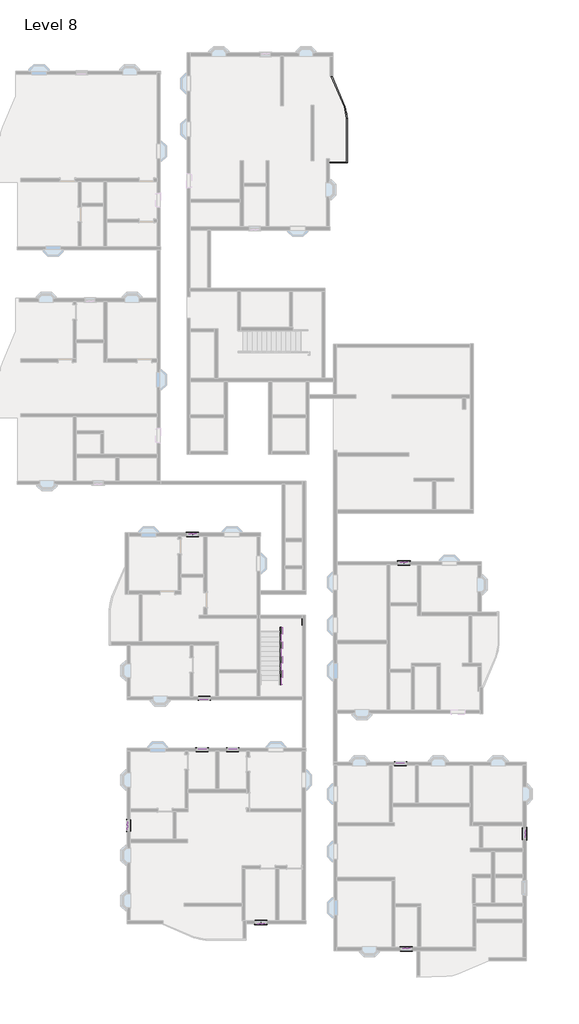
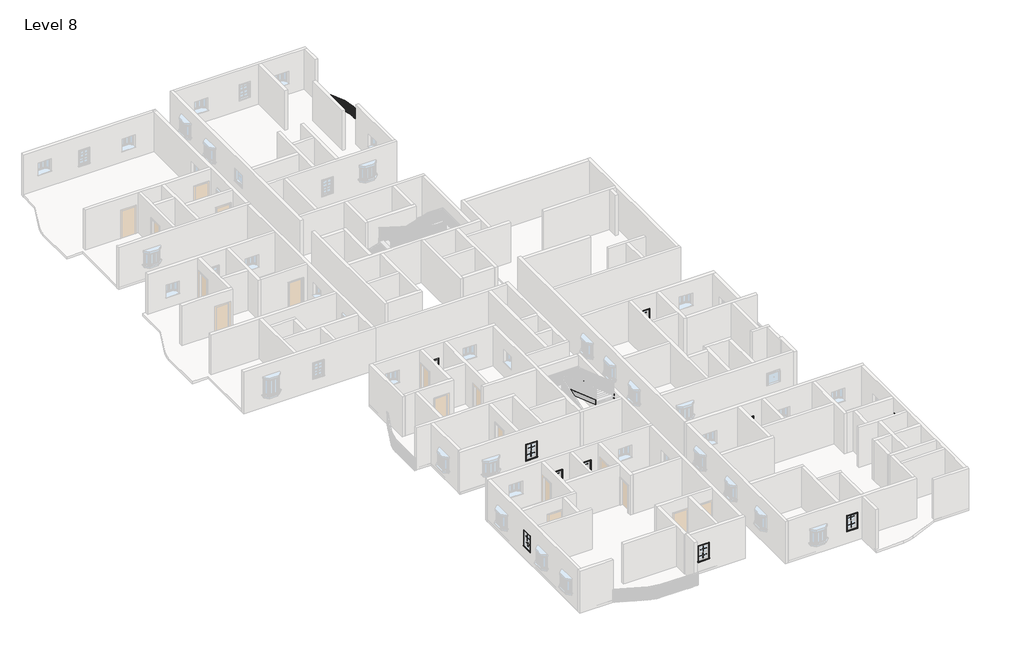
# One storey, part 13 of 14: 40 proxies, 6 members, 1 railing.
"""IFC4 building model written with IfcOpenShell, lengths in millimetres."""

from ifc_helpers import new_model, si_unit, frame, origin, place, context, project, spatial, polyline, circle_curve, outline, extrude, transform, mapped, element, save
from ifc_brep_helpers import plane_surface, cylinder_surface, revolved_surface, advanced_brep
from components import muntin_pattern_2x2_muntin_pattern_2x2_c35c595f, trim_window_exterior_flat_with_sill_e38017c9, trim_window_interior_flat_picture_frame_d728ed12

model = new_model("IFC4")

# Units and contexts
model_context = context("Model", 3, world=origin())
ifc_project = project(units=[si_unit("LENGTHUNIT", "METRE", prefix="MILLI")], contexts=[model_context])

# Site, building, storey
site = spatial("IfcSite", under=ifc_project)
building = spatial("IfcBuilding", under=site)
storey = spatial("IfcBuildingStorey", under=building, Name="Level 8", Elevation=21336.0)

# Proxies
placement = place(None, origin())
muntin_pattern_2x2_muntin_pattern_2x2_shape = muntin_pattern_2x2_muntin_pattern_2x2_c35c595f(model_context)
element("IfcBuildingElementProxy", 1, Name="Muntin Pattern_2x2 : Muntin Pattern_2x2", ObjectType="Muntin Pattern_2x2 : Muntin Pattern_2x2", at=placement, inside=storey, context=model_context, shape_type="MappedRepresentation", body=[
    mapped(muntin_pattern_2x2_muntin_pattern_2x2_shape, transform((-8150.287215, -357.5666506, 22806.025), x_axis=(1.0, 0.0, 0.0), y_axis=(0.0, 1.0, 0.0), z_axis=(0.0, 0.0, 1.0))),
])
element("IfcBuildingElementProxy", 2, Name="Muntin Pattern_2x2 : Muntin Pattern_2x2", ObjectType="Muntin Pattern_2x2 : Muntin Pattern_2x2", at=placement, inside=storey, context=model_context, shape_type="MappedRepresentation", body=[
    mapped(muntin_pattern_2x2_muntin_pattern_2x2_shape, transform((-8150.287215, -402.0166506, 22326.6), x_axis=(1.0, 0.0, 0.0), y_axis=(0.0, 1.0, 0.0), z_axis=(0.0, 0.0, 1.0))),
])
element("IfcBuildingElementProxy", 3, Name="Muntin Pattern_2x2 : Muntin Pattern_2x2", ObjectType="Muntin Pattern_2x2 : Muntin Pattern_2x2", at=placement, inside=storey, context=model_context, shape_type="MappedRepresentation", body=[
    mapped(muntin_pattern_2x2_muntin_pattern_2x2_shape, transform((-7397.812215, -10854.1166506, 22806.025), x_axis=(-1.0, 0.0, 0.0), y_axis=(0.0, -1.0, 0.0), z_axis=(0.0, 0.0, 1.0))),
])
element("IfcBuildingElementProxy", 4, Name="Muntin Pattern_2x2 : Muntin Pattern_2x2", ObjectType="Muntin Pattern_2x2 : Muntin Pattern_2x2", at=placement, inside=storey, context=model_context, shape_type="MappedRepresentation", body=[
    mapped(muntin_pattern_2x2_muntin_pattern_2x2_shape, transform((-7397.812215, -10809.6666506, 22326.6), x_axis=(-1.0, 0.0, 0.0), y_axis=(0.0, -1.0, 0.0), z_axis=(0.0, 0.0, 1.0))),
])
element("IfcBuildingElementProxy", 5, Name="Muntin Pattern_2x2 : Muntin Pattern_2x2", ObjectType="Muntin Pattern_2x2 : Muntin Pattern_2x2", at=placement, inside=storey, context=model_context, shape_type="MappedRepresentation", body=[
    mapped(muntin_pattern_2x2_muntin_pattern_2x2_shape, transform((-7540.687215, -13997.3666506, 22806.025), x_axis=(1.0, 0.0, 0.0), y_axis=(0.0, 1.0, 0.0), z_axis=(0.0, 0.0, 1.0))),
])
element("IfcBuildingElementProxy", 6, Name="Muntin Pattern_2x2 : Muntin Pattern_2x2", ObjectType="Muntin Pattern_2x2 : Muntin Pattern_2x2", at=placement, inside=storey, context=model_context, shape_type="MappedRepresentation", body=[
    mapped(muntin_pattern_2x2_muntin_pattern_2x2_shape, transform((-7540.687215, -14041.8166506, 22326.6), x_axis=(1.0, 0.0, 0.0), y_axis=(0.0, 1.0, 0.0), z_axis=(0.0, 0.0, 1.0))),
])
element("IfcBuildingElementProxy", 7, Name="Muntin Pattern_2x2 : Muntin Pattern_2x2", ObjectType="Muntin Pattern_2x2 : Muntin Pattern_2x2", at=placement, inside=storey, context=model_context, shape_type="MappedRepresentation", body=[
    mapped(muntin_pattern_2x2_muntin_pattern_2x2_shape, transform((-5597.587215, -13997.3666506, 22806.025), x_axis=(1.0, 0.0, 0.0), y_axis=(0.0, 1.0, 0.0), z_axis=(0.0, 0.0, 1.0))),
])
element("IfcBuildingElementProxy", 8, Name="Muntin Pattern_2x2 : Muntin Pattern_2x2", ObjectType="Muntin Pattern_2x2 : Muntin Pattern_2x2", at=placement, inside=storey, context=model_context, shape_type="MappedRepresentation", body=[
    mapped(muntin_pattern_2x2_muntin_pattern_2x2_shape, transform((-5597.587215, -14041.8166506, 22326.6), x_axis=(1.0, 0.0, 0.0), y_axis=(0.0, 1.0, 0.0), z_axis=(0.0, 0.0, 1.0))),
])
element("IfcBuildingElementProxy", 9, Name="Muntin Pattern_2x2 : Muntin Pattern_2x2", ObjectType="Muntin Pattern_2x2 : Muntin Pattern_2x2", at=placement, inside=storey, context=model_context, shape_type="MappedRepresentation", body=[
    mapped(muntin_pattern_2x2_muntin_pattern_2x2_shape, transform((-12255.562215, -18863.6994419, 22806.025), x_axis=(0.0, 1.0, 0.0), y_axis=(-1.0, 0.0, 0.0), z_axis=(0.0, 0.0, 1.0))),
])
element("IfcBuildingElementProxy", 10, Name="Muntin Pattern_2x2 : Muntin Pattern_2x2", ObjectType="Muntin Pattern_2x2 : Muntin Pattern_2x2", at=placement, inside=storey, context=model_context, shape_type="MappedRepresentation", body=[
    mapped(muntin_pattern_2x2_muntin_pattern_2x2_shape, transform((-12211.112215, -18863.6994419, 22326.6), x_axis=(0.0, 1.0, 0.0), y_axis=(-1.0, 0.0, 0.0), z_axis=(0.0, 0.0, 1.0))),
])
element("IfcBuildingElementProxy", 11, Name="Muntin Pattern_2x2 : Muntin Pattern_2x2", ObjectType="Muntin Pattern_2x2 : Muntin Pattern_2x2", at=placement, inside=storey, context=model_context, shape_type="MappedRepresentation", body=[
    mapped(muntin_pattern_2x2_muntin_pattern_2x2_shape, transform((-3806.2891351, -25065.4166506, 22806.025), x_axis=(-1.0, 0.0, 0.0), y_axis=(0.0, -1.0, 0.0), z_axis=(0.0, 0.0, 1.0))),
])
element("IfcBuildingElementProxy", 12, Name="Muntin Pattern_2x2 : Muntin Pattern_2x2", ObjectType="Muntin Pattern_2x2 : Muntin Pattern_2x2", at=placement, inside=storey, context=model_context, shape_type="MappedRepresentation", body=[
    mapped(muntin_pattern_2x2_muntin_pattern_2x2_shape, transform((-3806.2891351, -25020.9666506, 22326.6), x_axis=(-1.0, 0.0, 0.0), y_axis=(0.0, -1.0, 0.0), z_axis=(0.0, 0.0, 1.0))),
])
element("IfcBuildingElementProxy", 13, Name="Muntin Pattern_2x2 : Muntin Pattern_2x2", ObjectType="Muntin Pattern_2x2 : Muntin Pattern_2x2", at=placement, inside=storey, context=model_context, shape_type="MappedRepresentation", body=[
    mapped(muntin_pattern_2x2_muntin_pattern_2x2_shape, transform((5410.0380523, -26615.6292694, 22806.025), x_axis=(1.0, 0.0, 0.0), y_axis=(0.0, 1.0, 0.0), z_axis=(0.0, 0.0, 1.0))),
])
element("IfcBuildingElementProxy", 14, Name="Muntin Pattern_2x2 : Muntin Pattern_2x2", ObjectType="Muntin Pattern_2x2 : Muntin Pattern_2x2", at=placement, inside=storey, context=model_context, shape_type="MappedRepresentation", body=[
    mapped(muntin_pattern_2x2_muntin_pattern_2x2_shape, transform((5410.0380523, -26660.0792694, 22326.6), x_axis=(1.0, 0.0, 0.0), y_axis=(0.0, 1.0, 0.0), z_axis=(0.0, 0.0, 1.0))),
])
element("IfcBuildingElementProxy", 15, Name="Muntin Pattern_2x2 : Muntin Pattern_2x2", ObjectType="Muntin Pattern_2x2 : Muntin Pattern_2x2", at=placement, inside=storey, context=model_context, shape_type="MappedRepresentation", body=[
    mapped(muntin_pattern_2x2_muntin_pattern_2x2_shape, transform((12982.4130523, -19379.8042694, 22806.025), x_axis=(0.0, -1.0, 0.0), y_axis=(1.0, 0.0, 0.0), z_axis=(0.0, 0.0, 1.0))),
])
element("IfcBuildingElementProxy", 16, Name="Muntin Pattern_2x2 : Muntin Pattern_2x2", ObjectType="Muntin Pattern_2x2 : Muntin Pattern_2x2", at=placement, inside=storey, context=model_context, shape_type="MappedRepresentation", body=[
    mapped(muntin_pattern_2x2_muntin_pattern_2x2_shape, transform((12937.9630523, -19379.8042694, 22326.6), x_axis=(0.0, -1.0, 0.0), y_axis=(1.0, 0.0, 0.0), z_axis=(0.0, 0.0, 1.0))),
])
element("IfcBuildingElementProxy", 17, Name="Muntin Pattern_2x2 : Muntin Pattern_2x2", ObjectType="Muntin Pattern_2x2 : Muntin Pattern_2x2", at=placement, inside=storey, context=model_context, shape_type="MappedRepresentation", body=[
    mapped(muntin_pattern_2x2_muntin_pattern_2x2_shape, transform((5048.0880523, -14880.8292694, 22806.025), x_axis=(1.0, 0.0, 0.0), y_axis=(0.0, 1.0, 0.0), z_axis=(0.0, 0.0, 1.0))),
])
element("IfcBuildingElementProxy", 18, Name="Muntin Pattern_2x2 : Muntin Pattern_2x2", ObjectType="Muntin Pattern_2x2 : Muntin Pattern_2x2", at=placement, inside=storey, context=model_context, shape_type="MappedRepresentation", body=[
    mapped(muntin_pattern_2x2_muntin_pattern_2x2_shape, transform((5048.0880523, -14925.2792694, 22326.6), x_axis=(1.0, 0.0, 0.0), y_axis=(0.0, 1.0, 0.0), z_axis=(0.0, 0.0, 1.0))),
])
element("IfcBuildingElementProxy", 19, Name="Muntin Pattern_2x2 : Muntin Pattern_2x2", ObjectType="Muntin Pattern_2x2 : Muntin Pattern_2x2", at=placement, inside=storey, context=model_context, shape_type="MappedRepresentation", body=[
    mapped(muntin_pattern_2x2_muntin_pattern_2x2_shape, transform((5257.6380523, -2168.1292694, 22806.025), x_axis=(1.0, 0.0, 0.0), y_axis=(0.0, 1.0, 0.0), z_axis=(0.0, 0.0, 1.0))),
])
element("IfcBuildingElementProxy", 20, Name="Muntin Pattern_2x2 : Muntin Pattern_2x2", ObjectType="Muntin Pattern_2x2 : Muntin Pattern_2x2", at=placement, inside=storey, context=model_context, shape_type="MappedRepresentation", body=[
    mapped(muntin_pattern_2x2_muntin_pattern_2x2_shape, transform((5257.6380523, -2212.5792694, 22326.6), x_axis=(1.0, 0.0, 0.0), y_axis=(0.0, 1.0, 0.0), z_axis=(0.0, 0.0, 1.0))),
])
trim_window_exterior_flat_with_sill_shape = trim_window_exterior_flat_with_sill_e38017c9(model_context)
element("IfcBuildingElementProxy", 21, Name="Trim-Window-Exterior-Flat : with Sill", ObjectType="Trim-Window-Exterior-Flat : with Sill", at=placement, inside=storey, context=model_context, shape_type="MappedRepresentation", body=[
    mapped(trim_window_exterior_flat_with_sill_shape, transform((-8150.287215, -322.6416506, 23317.2), x_axis=(-1.0, 0.0, 0.0), y_axis=(0.0, 0.0, 1.0), z_axis=(0.0, 1.0, 0.0))),
])
element("IfcBuildingElementProxy", 22, Name="Trim-Window-Exterior-Flat : with Sill", ObjectType="Trim-Window-Exterior-Flat : with Sill", at=placement, inside=storey, context=model_context, shape_type="MappedRepresentation", body=[
    mapped(trim_window_exterior_flat_with_sill_shape, transform((-7397.812215, -10889.0416506, 23317.2), x_axis=(1.0, 0.0, 0.0), y_axis=(0.0, 0.0, 1.0), z_axis=(0.0, -1.0, 0.0))),
])
element("IfcBuildingElementProxy", 23, Name="Trim-Window-Exterior-Flat : with Sill", ObjectType="Trim-Window-Exterior-Flat : with Sill", at=placement, inside=storey, context=model_context, shape_type="MappedRepresentation", body=[
    mapped(trim_window_exterior_flat_with_sill_shape, transform((-7540.687215, -13962.4416506, 23317.2), x_axis=(-1.0, 0.0, 0.0), y_axis=(0.0, 0.0, 1.0), z_axis=(0.0, 1.0, 0.0))),
])
element("IfcBuildingElementProxy", 24, Name="Trim-Window-Exterior-Flat : with Sill", ObjectType="Trim-Window-Exterior-Flat : with Sill", at=placement, inside=storey, context=model_context, shape_type="MappedRepresentation", body=[
    mapped(trim_window_exterior_flat_with_sill_shape, transform((-5597.587215, -13962.4416506, 23317.2), x_axis=(-1.0, 0.0, 0.0), y_axis=(0.0, 0.0, 1.0), z_axis=(0.0, 1.0, 0.0))),
])
element("IfcBuildingElementProxy", 25, Name="Trim-Window-Exterior-Flat : with Sill", ObjectType="Trim-Window-Exterior-Flat : with Sill", at=placement, inside=storey, context=model_context, shape_type="MappedRepresentation", body=[
    mapped(trim_window_exterior_flat_with_sill_shape, transform((-12290.487215, -18863.6994419, 23317.2), x_axis=(0.0, -1.0, 0.0), y_axis=(0.0, 0.0, 1.0), z_axis=(-1.0, 0.0, 0.0))),
])
element("IfcBuildingElementProxy", 26, Name="Trim-Window-Exterior-Flat : with Sill", ObjectType="Trim-Window-Exterior-Flat : with Sill", at=placement, inside=storey, context=model_context, shape_type="MappedRepresentation", body=[
    mapped(trim_window_exterior_flat_with_sill_shape, transform((-3806.2891351, -25100.3416506, 23317.2), x_axis=(1.0, 0.0, 0.0), y_axis=(0.0, 0.0, 1.0), z_axis=(0.0, -1.0, 0.0))),
])
element("IfcBuildingElementProxy", 27, Name="Trim-Window-Exterior-Flat : with Sill", ObjectType="Trim-Window-Exterior-Flat : with Sill", at=placement, inside=storey, context=model_context, shape_type="MappedRepresentation", body=[
    mapped(trim_window_exterior_flat_with_sill_shape, transform((5410.0380523, -26580.7042694, 23317.2), x_axis=(-1.0, 0.0, 0.0), y_axis=(0.0, 0.0, 1.0), z_axis=(0.0, 1.0, 0.0))),
])
element("IfcBuildingElementProxy", 28, Name="Trim-Window-Exterior-Flat : with Sill", ObjectType="Trim-Window-Exterior-Flat : with Sill", at=placement, inside=storey, context=model_context, shape_type="MappedRepresentation", body=[
    mapped(trim_window_exterior_flat_with_sill_shape, transform((13017.3380523, -19379.8042694, 23317.2), x_axis=(0.0, 1.0, 0.0), y_axis=(0.0, 0.0, 1.0), z_axis=(1.0, 0.0, 0.0))),
])
element("IfcBuildingElementProxy", 29, Name="Trim-Window-Exterior-Flat : with Sill", ObjectType="Trim-Window-Exterior-Flat : with Sill", at=placement, inside=storey, context=model_context, shape_type="MappedRepresentation", body=[
    mapped(trim_window_exterior_flat_with_sill_shape, transform((5048.0880523, -14845.9042694, 23317.2), x_axis=(-1.0, 0.0, 0.0), y_axis=(0.0, 0.0, 1.0), z_axis=(0.0, 1.0, 0.0))),
])
element("IfcBuildingElementProxy", 30, Name="Trim-Window-Exterior-Flat : with Sill", ObjectType="Trim-Window-Exterior-Flat : with Sill", at=placement, inside=storey, context=model_context, shape_type="MappedRepresentation", body=[
    mapped(trim_window_exterior_flat_with_sill_shape, transform((5257.6380523, -2133.2042694, 23317.2), x_axis=(-1.0, 0.0, 0.0), y_axis=(0.0, 0.0, 1.0), z_axis=(0.0, 1.0, 0.0))),
])
trim_window_interior_flat_picture_frame_shape = trim_window_interior_flat_picture_frame_d728ed12(model_context)
element("IfcBuildingElementProxy", 31, Name="Trim-Window-Interior-Flat : Picture Frame", ObjectType="Trim-Window-Interior-Flat : Picture Frame", at=placement, inside=storey, context=model_context, shape_type="MappedRepresentation", body=[
    mapped(trim_window_interior_flat_picture_frame_shape, transform((-8150.287215, -525.8416506, 23317.2), x_axis=(1.0, 0.0, 0.0), y_axis=(0.0, 0.0, 1.0), z_axis=(0.0, -1.0, 0.0))),
])
element("IfcBuildingElementProxy", 32, Name="Trim-Window-Interior-Flat : Picture Frame", ObjectType="Trim-Window-Interior-Flat : Picture Frame", at=placement, inside=storey, context=model_context, shape_type="MappedRepresentation", body=[
    mapped(trim_window_interior_flat_picture_frame_shape, transform((-7397.812215, -10685.8416506, 23317.2), x_axis=(-1.0, 0.0, 0.0), y_axis=(0.0, 0.0, 1.0), z_axis=(0.0, 1.0, 0.0))),
])
element("IfcBuildingElementProxy", 33, Name="Trim-Window-Interior-Flat : Picture Frame", ObjectType="Trim-Window-Interior-Flat : Picture Frame", at=placement, inside=storey, context=model_context, shape_type="MappedRepresentation", body=[
    mapped(trim_window_interior_flat_picture_frame_shape, transform((-7540.687215, -14165.6416506, 23317.2), x_axis=(1.0, 0.0, 0.0), y_axis=(0.0, 0.0, 1.0), z_axis=(0.0, -1.0, 0.0))),
])
element("IfcBuildingElementProxy", 34, Name="Trim-Window-Interior-Flat : Picture Frame", ObjectType="Trim-Window-Interior-Flat : Picture Frame", at=placement, inside=storey, context=model_context, shape_type="MappedRepresentation", body=[
    mapped(trim_window_interior_flat_picture_frame_shape, transform((-5597.587215, -14165.6416506, 23317.2), x_axis=(1.0, 0.0, 0.0), y_axis=(0.0, 0.0, 1.0), z_axis=(0.0, -1.0, 0.0))),
])
element("IfcBuildingElementProxy", 35, Name="Trim-Window-Interior-Flat : Picture Frame", ObjectType="Trim-Window-Interior-Flat : Picture Frame", at=placement, inside=storey, context=model_context, shape_type="MappedRepresentation", body=[
    mapped(trim_window_interior_flat_picture_frame_shape, transform((-12087.287215, -18863.6994419, 23317.2), x_axis=(0.0, 1.0, 0.0), y_axis=(0.0, 0.0, 1.0), z_axis=(1.0, 0.0, 0.0))),
])
element("IfcBuildingElementProxy", 36, Name="Trim-Window-Interior-Flat : Picture Frame", ObjectType="Trim-Window-Interior-Flat : Picture Frame", at=placement, inside=storey, context=model_context, shape_type="MappedRepresentation", body=[
    mapped(trim_window_interior_flat_picture_frame_shape, transform((-3806.2891351, -24897.1416506, 23317.2), x_axis=(-1.0, 0.0, 0.0), y_axis=(0.0, 0.0, 1.0), z_axis=(0.0, 1.0, 0.0))),
])
element("IfcBuildingElementProxy", 37, Name="Trim-Window-Interior-Flat : Picture Frame", ObjectType="Trim-Window-Interior-Flat : Picture Frame", at=placement, inside=storey, context=model_context, shape_type="MappedRepresentation", body=[
    mapped(trim_window_interior_flat_picture_frame_shape, transform((5410.0380523, -26783.9042694, 23317.2), x_axis=(1.0, 0.0, 0.0), y_axis=(0.0, 0.0, 1.0), z_axis=(0.0, -1.0, 0.0))),
])
element("IfcBuildingElementProxy", 38, Name="Trim-Window-Interior-Flat : Picture Frame", ObjectType="Trim-Window-Interior-Flat : Picture Frame", at=placement, inside=storey, context=model_context, shape_type="MappedRepresentation", body=[
    mapped(trim_window_interior_flat_picture_frame_shape, transform((12814.1380523, -19379.8042694, 23317.2), x_axis=(0.0, -1.0, 0.0), y_axis=(0.0, 0.0, 1.0), z_axis=(-1.0, 0.0, 0.0))),
])
element("IfcBuildingElementProxy", 39, Name="Trim-Window-Interior-Flat : Picture Frame", ObjectType="Trim-Window-Interior-Flat : Picture Frame", at=placement, inside=storey, context=model_context, shape_type="MappedRepresentation", body=[
    mapped(trim_window_interior_flat_picture_frame_shape, transform((5048.0880523, -15049.1042694, 23317.2), x_axis=(1.0, 0.0, 0.0), y_axis=(0.0, 0.0, 1.0), z_axis=(0.0, -1.0, 0.0))),
])
element("IfcBuildingElementProxy", 40, Name="Trim-Window-Interior-Flat : Picture Frame", ObjectType="Trim-Window-Interior-Flat : Picture Frame", at=placement, inside=storey, context=model_context, shape_type="MappedRepresentation", body=[
    mapped(trim_window_interior_flat_picture_frame_shape, transform((5257.6380523, -2336.4042694, 23317.2), x_axis=(1.0, 0.0, 0.0), y_axis=(0.0, 0.0, 1.0), z_axis=(0.0, -1.0, 0.0))),
])

# Members
element("IfcMember", 41, ObjectType="Stringer - 2\" Width", at=placement, inside=storey, context=model_context, shape_type="SweptSolid", body=[
    extrude(outline(polyline([(-9955.5916506, 21336.0), (-9955.5916506, 21527.3592169), (-6325.8738327, 22783.8), (-5713.7916506, 22783.8), (-5713.7916506, 22673.1301656), (-9576.612129, 21336.0), (-9955.5916506, 21336.0)])), frame((-3908.487215, 0.0, 0.0), z_axis=(1.0, 0.0, 0.0), x_axis=(0.0, 1.0, 0.0)), (0.0, 0.0, 1.0), 50.8),
])
element("IfcMember", 42, ObjectType="Stringer - 2\" Width", at=placement, inside=storey, context=model_context, shape_type="SweptSolid", body=[
    extrude(outline(polyline([(-3908.487215, -5713.7916506), (-3908.487215, -5662.9916506), (-1190.687215, -5662.9916506), (-1190.687215, -5713.7916506), (-3908.487215, -5713.7916506)])), frame((0.0, 0.0, 22479.0), z_axis=(0.0, 0.0, 1.0), x_axis=(1.0, 0.0, 0.0)), (0.0, 0.0, 1.0), 304.8),
])
element("IfcMember", 43, ObjectType="Stringer - 2\" Width", at=placement, inside=storey, context=model_context, shape_type="SweptSolid", body=[
    extrude(outline(polyline([(-5662.9916506, 22683.5476784), (-5662.9916506, 22479.0), (-6003.8711722, 22479.0), (-9949.2416506, 23844.7051656), (-9949.2416506, 24167.2496015), (-5662.9916506, 22683.5476784)])), frame((-1190.687215, 0.0, 0.0), z_axis=(1.0, 0.0, 0.0), x_axis=(0.0, 1.0, 0.0)), (0.0, 0.0, 1.0), 50.8),
])
element("IfcMember", 44, ObjectType="Stringer - 2\" Width", at=placement, inside=storey, context=model_context, shape_type="SweptSolid", body=[
    extrude(outline(polyline([(-9955.5916506, 21336.0), (-9955.5916506, 21527.3592169), (-6342.4416506, 22778.0649861), (-6342.4416506, 22455.5205502), (-9576.612129, 21336.0), (-9955.5916506, 21336.0)])), frame((-2593.7381751, 0.0, 0.0), z_axis=(1.0, 0.0, 0.0), x_axis=(0.0, 1.0, 0.0)), (0.0, 0.0, 1.0), 50.8),
])
element("IfcMember", 45, ObjectType="Stringer - 2\" Width", at=placement, inside=storey, context=model_context, shape_type="SweptSolid", body=[
    extrude(outline(polyline([(-2593.7381751, -6342.4416506), (-2593.7381751, -6291.6416506), (-2492.1381751, -6291.6416506), (-2492.1381751, -6342.4416506), (-2593.7381751, -6342.4416506)])), frame((0.0, 0.0, 22479.0), z_axis=(0.0, 0.0, 1.0), x_axis=(1.0, 0.0, 0.0)), (0.0, 0.0, 1.0), 304.8),
])
element("IfcMember", 46, ObjectType="Stringer - 2\" Width", at=placement, inside=storey, context=model_context, shape_type="SweptSolid", body=[
    extrude(outline(polyline([(-6291.6416506, 22901.1572938), (-6291.6416506, 22578.6128579), (-9949.2416506, 23844.7051656), (-9949.2416506, 24167.2496015), (-6291.6416506, 22901.1572938)])), frame((-2492.1381751, 0.0, 0.0), z_axis=(1.0, 0.0, 0.0), x_axis=(0.0, 1.0, 0.0)), (0.0, 0.0, 1.0), 50.8),
])

# Railing
element("IfcRailing", 47, ObjectType="Handrail - Rectangular", at=placement, inside=storey, context=model_context, shape_type="SolidModel", body=[
    advanced_brep(
    [(549.8108649, 23180.4215905, 22250.4), (549.8108649, 23180.4215905, 22199.6), (549.8108649, 23129.6215905, 22199.6), (549.8108649, 23129.6215905, 22250.4), (1629.3108649, 23180.4215905, 22250.4), (1629.3108649, 23180.4215905, 22199.6), (1680.1108649, 23129.6215905, 22199.6), (1680.1108649, 23129.6215905, 22250.4), (1629.3108649, 25921.9580583, 22250.4), (1629.3108649, 25921.9580583, 22199.6), (1680.1108649, 25921.9580583, 22199.6), (1680.1108649, 25921.9580583, 22250.4), (1475.5051478, 26671.8537734, 22199.6), (1475.5051478, 26671.8537734, 22250.4), (1522.203662, 26691.8509925, 22199.6), (1522.203662, 26691.8509925, 22250.4), (640.7616078, 28621.188975, 22250.4), (687.460122, 28641.186194, 22250.4), (687.460122, 28641.186194, 22199.6), (640.7616078, 28621.188975, 22199.6)],
    [
        (0, 1),
        (1, 2),
        (2, 3),
        (3, 0),
        (0, 4),
        (4, 5),
        (5, 1),
        (5, 6),
        (6, 2),
        (6, 7),
        (7, 3),
        (7, 4),
        (4, 8),
        (8, 9),
        (9, 5),
        (9, 10),
        (10, 6),
        (10, 11),
        (11, 7),
        (11, 8),
        (12, 9, circle_curve(frame((-275.6891351, 25921.9580583, 22199.6), z_axis=(0.0, 0.0, -1.0), x_axis=(1.0, 0.0, 0.0)), 1905.0)),
        (8, 13, circle_curve(frame((-275.6891351, 25921.9580583, 22250.4), z_axis=(0.0, 0.0, 1.0), x_axis=(1.0, 0.0, 0.0)), 1905.0)),
        (13, 12),
        (14, 10, circle_curve(frame((-275.6891351, 25921.9580583, 22199.6), z_axis=(0.0, 0.0, -1.0), x_axis=(1.0, 0.0, 0.0)), 1955.8)),
        (12, 14),
        (15, 11, circle_curve(frame((-275.6891351, 25921.9580583, 22250.4), z_axis=(0.0, 0.0, -1.0), x_axis=(1.0, 0.0, 0.0)), 1955.8)),
        (14, 15),
        (15, 13),
        (16, 17),
        (17, 18),
        (18, 19),
        (19, 16),
        (13, 16),
        (19, 12),
        (18, 14),
        (17, 15),
    ],
    [
        plane_surface(frame((549.8108649, 23155.0215905, 22250.4), z_axis=(-1.0, 0.0, 0.0), x_axis=(0.0, 1.0, 0.0))),
        plane_surface(frame((549.8108649, 23180.4215905, 22250.4), z_axis=(0.0, 1.0, 0.0), x_axis=(1.0, 0.0, 0.0))),
        plane_surface(frame((549.8108649, 23180.4215905, 22199.6), z_axis=(0.0, 0.0, -1.0), x_axis=(1.0, 0.0, 0.0))),
        plane_surface(frame((549.8108649, 23129.6215905, 22199.6), z_axis=(0.0, -1.0, 0.0), x_axis=(1.0, 0.0, 0.0))),
        plane_surface(frame((549.8108649, 23129.6215905, 22250.4), z_axis=(0.0, 0.0, 1.0), x_axis=(1.0, 0.0, 0.0))),
        plane_surface(frame((1629.3108649, 23180.4215905, 22250.4), z_axis=(-1.0, 0.0, 0.0), x_axis=(0.0, 1.0, 0.0))),
        plane_surface(frame((1629.3108649, 23180.4215905, 22199.6), z_axis=(0.0, 0.0, -1.0), x_axis=(0.0, 1.0, 0.0))),
        plane_surface(frame((1680.1108649, 23129.6215905, 22199.6), z_axis=(1.0, 0.0, 0.0), x_axis=(0.0, 1.0, 0.0))),
        plane_surface(frame((1680.1108649, 23129.6215905, 22250.4), z_axis=(0.0, 0.0, 1.0), x_axis=(0.0, 1.0, 0.0))),
        revolved_surface(polyline([(1629.3108649, 25921.9580583, 22250.4), (1629.3108649, 25921.9580583, 22199.6)]), (-275.6891351, 25921.9580583, 22250.4), (0.0, 0.0, 1.0)),
        plane_surface(frame((-275.6891351, 25921.9580583, 22199.6), z_axis=(0.0, 0.0, -1.0), x_axis=(1.0, 0.0, 0.0))),
        cylinder_surface(frame((-275.6891351, 25921.9580583, 22250.4), z_axis=(0.0, 0.0, 1.0), x_axis=(1.0, 0.0, 0.0)), 1955.8),
        plane_surface(frame((-275.6891351, 25921.9580583, 22250.4), z_axis=(0.0, 0.0, 1.0), x_axis=(1.0, 0.0, 0.0))),
        plane_surface(frame((664.1108649, 28631.1875845, 22250.4), z_axis=(-0.39364604467361036, 0.91926209076238, 0.0), x_axis=(0.91926209076238, 0.39364604467361036, 0.0))),
        plane_surface(frame((1475.5051478, 26671.8537734, 22250.4), z_axis=(-0.9192620907623801, -0.39364604467361, 0.0), x_axis=(-0.39364604467361, 0.9192620907623801, 0.0))),
        plane_surface(frame((1475.5051478, 26671.8537734, 22199.6), z_axis=(0.0, 0.0, -1.0), x_axis=(-0.39364604467361, 0.9192620907623801, 0.0))),
        plane_surface(frame((1522.203662, 26691.8509925, 22199.6), z_axis=(0.91926209076238, 0.3936460446736103, 0.0), x_axis=(-0.3936460446736103, 0.91926209076238, 0.0))),
        plane_surface(frame((1522.203662, 26691.8509925, 22250.4), z_axis=(0.0, 0.0, 1.0000000000000002), x_axis=(-0.3936460446736103, 0.91926209076238, 0.0))),
    ],
    [
        (0, [[1, 2, 3, 4]]),
        (1, [[-1, 5, 6, 7]]),
        (2, [[-2, -7, 8, 9]]),
        (3, [[-3, -9, 10, 11]]),
        (4, [[-4, -11, 12, -5]]),
        (5, [[-6, 13, 14, 15]]),
        (6, [[-8, -15, 16, 17]]),
        (7, [[-10, -17, 18, 19]]),
        (8, [[-12, -19, 20, -13]]),
        (9, [[21, -14, 22, 23]]),
        (10, [[24, -16, -21, 25]]),
        (11, [[26, -18, -24, 27]]),
        (12, [[-22, -20, -26, 28]]),
        (13, [[29, 30, 31, 32]]),
        (14, [[-23, 33, -32, 34]]),
        (15, [[-25, -34, -31, 35]]),
        (16, [[-27, -35, -30, 36]]),
        (17, [[-28, -36, -29, -33]]),
    ],
),
    extrude(outline(polyline([(711.4710921, 28544.7864585), (693.9591493, 28537.2875014), (686.4601921, 28554.7994442), (703.9721349, 28562.2984014), (711.4710921, 28544.7864585)])), frame((0.0, 0.0, 21336.0), z_axis=(0.0, 0.0, 1.0), x_axis=(1.0, 0.0, 0.0)), (0.0, 0.0, 1.0), 863.6),
    extrude(outline(polyline([(751.4655302, 28451.3894301), (733.9535874, 28443.890473), (726.4546303, 28461.4024158), (743.9665731, 28468.9013729), (751.4655302, 28451.3894301)])), frame((0.0, 0.0, 21336.0), z_axis=(0.0, 0.0, 1.0), x_axis=(1.0, 0.0, 0.0)), (0.0, 0.0, 1.0), 863.6),
    extrude(outline(polyline([(791.4599684, 28357.9924017), (773.9480255, 28350.4934445), (766.4490684, 28368.0053874), (783.9610112, 28375.5043445), (791.4599684, 28357.9924017)])), frame((0.0, 0.0, 21336.0), z_axis=(0.0, 0.0, 1.0), x_axis=(1.0, 0.0, 0.0)), (0.0, 0.0, 1.0), 863.6),
    extrude(outline(polyline([(831.4544065, 28264.5953733), (813.9424637, 28257.0964161), (806.4435065, 28274.608359), (823.9554494, 28282.1073161), (831.4544065, 28264.5953733)])), frame((0.0, 0.0, 21336.0), z_axis=(0.0, 0.0, 1.0), x_axis=(1.0, 0.0, 0.0)), (0.0, 0.0, 1.0), 863.6),
    extrude(outline(polyline([(871.4488446, 28171.1983449), (853.9369018, 28163.6993877), (846.4379447, 28181.2113305), (863.9498875, 28188.7102877), (871.4488446, 28171.1983449)])), frame((0.0, 0.0, 21336.0), z_axis=(0.0, 0.0, 1.0), x_axis=(1.0, 0.0, 0.0)), (0.0, 0.0, 1.0), 863.6),
    extrude(outline(polyline([(911.4432828, 28077.8013164), (893.93134, 28070.3023593), (886.4323828, 28087.8143021), (903.9443256, 28095.3132593), (911.4432828, 28077.8013164)])), frame((0.0, 0.0, 21336.0), z_axis=(0.0, 0.0, 1.0), x_axis=(1.0, 0.0, 0.0)), (0.0, 0.0, 1.0), 863.6),
    extrude(outline(polyline([(951.4377209, 27984.404288), (933.9257781, 27976.9053309), (926.4268209, 27994.4172737), (943.9387638, 28001.9162308), (951.4377209, 27984.404288)])), frame((0.0, 0.0, 21336.0), z_axis=(0.0, 0.0, 1.0), x_axis=(1.0, 0.0, 0.0)), (0.0, 0.0, 1.0), 863.6),
    extrude(outline(polyline([(991.4321591, 27891.0072596), (973.9202162, 27883.5083024), (966.4212591, 27901.0202453), (983.9332019, 27908.5192024), (991.4321591, 27891.0072596)])), frame((0.0, 0.0, 21336.0), z_axis=(0.0, 0.0, 1.0), x_axis=(1.0, 0.0, 0.0)), (0.0, 0.0, 1.0), 863.6),
    extrude(outline(polyline([(1031.4265972, 27797.6102312), (1013.9146544, 27790.111274), (1006.4156972, 27807.6232168), (1023.9276401, 27815.122174), (1031.4265972, 27797.6102312)])), frame((0.0, 0.0, 21336.0), z_axis=(0.0, 0.0, 1.0), x_axis=(1.0, 0.0, 0.0)), (0.0, 0.0, 1.0), 863.6),
    extrude(outline(polyline([(1071.4210353, 27704.2132027), (1053.9090925, 27696.7142456), (1046.4101354, 27714.2261884), (1063.9220782, 27721.7251456), (1071.4210353, 27704.2132027)])), frame((0.0, 0.0, 21336.0), z_axis=(0.0, 0.0, 1.0), x_axis=(1.0, 0.0, 0.0)), (0.0, 0.0, 1.0), 863.6),
    extrude(outline(polyline([(1111.4154735, 27610.8161743), (1093.9035307, 27603.3172172), (1086.4045735, 27620.82916), (1103.9165163, 27628.3281172), (1111.4154735, 27610.8161743)])), frame((0.0, 0.0, 21336.0), z_axis=(0.0, 0.0, 1.0), x_axis=(1.0, 0.0, 0.0)), (0.0, 0.0, 1.0), 863.6),
    extrude(outline(polyline([(1151.4099116, 27517.4191459), (1133.8979688, 27509.9201888), (1126.3990116, 27527.4321316), (1143.9109545, 27534.9310887), (1151.4099116, 27517.4191459)])), frame((0.0, 0.0, 21336.0), z_axis=(0.0, 0.0, 1.0), x_axis=(1.0, 0.0, 0.0)), (0.0, 0.0, 1.0), 863.6),
    extrude(outline(polyline([(1191.4043498, 27424.0221175), (1173.8924069, 27416.5231603), (1166.3934498, 27434.0351032), (1183.9053926, 27441.5340603), (1191.4043498, 27424.0221175)])), frame((0.0, 0.0, 21336.0), z_axis=(0.0, 0.0, 1.0), x_axis=(1.0, 0.0, 0.0)), (0.0, 0.0, 1.0), 863.6),
    extrude(outline(polyline([(1231.3987879, 27330.6250891), (1213.8868451, 27323.1261319), (1206.3878879, 27340.6380747), (1223.8998307, 27348.1370319), (1231.3987879, 27330.6250891)])), frame((0.0, 0.0, 21336.0), z_axis=(0.0, 0.0, 1.0), x_axis=(1.0, 0.0, 0.0)), (0.0, 0.0, 1.0), 863.6),
    extrude(outline(polyline([(1271.393226, 27237.2280606), (1253.8812832, 27229.7291035), (1246.3823261, 27247.2410463), (1263.8942689, 27254.7400035), (1271.393226, 27237.2280606)])), frame((0.0, 0.0, 21336.0), z_axis=(0.0, 0.0, 1.0), x_axis=(1.0, 0.0, 0.0)), (0.0, 0.0, 1.0), 863.6),
    extrude(outline(polyline([(1311.3876642, 27143.8310322), (1293.8757213, 27136.3320751), (1286.3767642, 27153.8440179), (1303.888707, 27161.342975), (1311.3876642, 27143.8310322)])), frame((0.0, 0.0, 21336.0), z_axis=(0.0, 0.0, 1.0), x_axis=(1.0, 0.0, 0.0)), (0.0, 0.0, 1.0), 863.6),
    extrude(outline(polyline([(1351.3821023, 27050.4340038), (1333.8701595, 27042.9350466), (1326.3712023, 27060.4469895), (1343.8831452, 27067.9459466), (1351.3821023, 27050.4340038)])), frame((0.0, 0.0, 21336.0), z_axis=(0.0, 0.0, 1.0), x_axis=(1.0, 0.0, 0.0)), (0.0, 0.0, 1.0), 863.6),
    extrude(outline(polyline([(1391.3765405, 26957.0369754), (1373.8645976, 26949.5380182), (1366.3656405, 26967.0499611), (1383.8775833, 26974.5489182), (1391.3765405, 26957.0369754)])), frame((0.0, 0.0, 21336.0), z_axis=(0.0, 0.0, 1.0), x_axis=(1.0, 0.0, 0.0)), (0.0, 0.0, 1.0), 863.6),
    extrude(outline(polyline([(1431.3709786, 26863.639947), (1413.8590358, 26856.1409898), (1406.3600786, 26873.6529326), (1423.8720214, 26881.1518898), (1431.3709786, 26863.639947)])), frame((0.0, 0.0, 21336.0), z_axis=(0.0, 0.0, 1.0), x_axis=(1.0, 0.0, 0.0)), (0.0, 0.0, 1.0), 863.6),
    extrude(outline(polyline([(1471.3654167, 26770.2429185), (1453.8534739, 26762.7439614), (1446.3545168, 26780.2559042), (1463.8664596, 26787.7548614), (1471.3654167, 26770.2429185)])), frame((0.0, 0.0, 21336.0), z_axis=(0.0, 0.0, 1.0), x_axis=(1.0, 0.0, 0.0)), (0.0, 0.0, 1.0), 863.6),
    extrude(outline(polyline([(1537.4917391, 26611.722401), (1519.7200483, 26604.8616791), (1512.8593263, 26622.6333699), (1530.6310171, 26629.4940918), (1537.4917391, 26611.722401)])), frame((0.0, 0.0, 21336.0), z_axis=(0.0, 0.0, 1.0), x_axis=(1.0, 0.0, 0.0)), (0.0, 0.0, 1.0), 863.6),
    extrude(outline(polyline([(1571.2676162, 26515.3807493), (1553.1596103, 26509.4644479), (1547.2433088, 26527.5724538), (1565.3513147, 26533.4887552), (1571.2676162, 26515.3807493)])), frame((0.0, 0.0, 21336.0), z_axis=(0.0, 0.0, 1.0), x_axis=(1.0, 0.0, 0.0)), (0.0, 0.0, 1.0), 863.6),
    extrude(outline(polyline([(1599.9284504, 26417.3956468), (1581.5342785, 26412.4401508), (1576.5787825, 26430.8343227), (1594.9729544, 26435.7898187), (1599.9284504, 26417.3956468)])), frame((0.0, 0.0, 21336.0), z_axis=(0.0, 0.0, 1.0), x_axis=(1.0, 0.0, 0.0)), (0.0, 0.0, 1.0), 863.6),
    extrude(outline(polyline([(1623.3948673, 26318.0384578), (1604.7654711, 26314.0574912), (1600.7845045, 26332.6868874), (1619.4139008, 26336.667854), (1623.3948673, 26318.0384578)])), frame((0.0, 0.0, 21336.0), z_axis=(0.0, 0.0, 1.0), x_axis=(1.0, 0.0, 0.0)), (0.0, 0.0, 1.0), 863.6),
    extrude(outline(polyline([(1641.601878, 26217.5843464), (1622.7888504, 26214.5889343), (1619.7934383, 26233.4019618), (1638.6064659, 26236.3973739), (1641.601878, 26217.5843464)])), frame((0.0, 0.0, 21336.0), z_axis=(0.0, 0.0, 1.0), x_axis=(1.0, 0.0, 0.0)), (0.0, 0.0, 1.0), 863.6),
    extrude(outline(polyline([(1654.4990591, 26116.3115146), (1635.5545019, 26114.3099526), (1633.5529398, 26133.2545098), (1652.4974971, 26135.2560719), (1654.4990591, 26116.3115146)])), frame((0.0, 0.0, 21336.0), z_axis=(0.0, 0.0, 1.0), x_axis=(1.0, 0.0, 0.0)), (0.0, 0.0, 1.0), 863.6),
    extrude(outline(polyline([(1662.0506927, 26014.5004319), (1643.0270716, 26013.4982632), (1642.0249029, 26032.5218842), (1661.048524, 26033.524053), (1662.0506927, 26014.5004319)])), frame((0.0, 0.0, 21336.0), z_axis=(0.0, 0.0, 1.0), x_axis=(1.0, 0.0, 0.0)), (0.0, 0.0, 1.0), 863.6),
    extrude(outline(polyline([(1664.2358649, 25888.6965905), (1645.1858649, 25888.6965905), (1645.1858649, 25907.7465905), (1664.2358649, 25907.7465905), (1664.2358649, 25888.6965905)])), frame((0.0, 0.0, 21336.0), z_axis=(0.0, 0.0, 1.0), x_axis=(1.0, 0.0, 0.0)), (0.0, 0.0, 1.0), 863.6),
    extrude(outline(polyline([(1664.2358649, 25787.0965905), (1645.1858649, 25787.0965905), (1645.1858649, 25806.1465905), (1664.2358649, 25806.1465905), (1664.2358649, 25787.0965905)])), frame((0.0, 0.0, 21336.0), z_axis=(0.0, 0.0, 1.0), x_axis=(1.0, 0.0, 0.0)), (0.0, 0.0, 1.0), 863.6),
    extrude(outline(polyline([(1664.2358649, 25685.4965905), (1645.1858649, 25685.4965905), (1645.1858649, 25704.5465905), (1664.2358649, 25704.5465905), (1664.2358649, 25685.4965905)])), frame((0.0, 0.0, 21336.0), z_axis=(0.0, 0.0, 1.0), x_axis=(1.0, 0.0, 0.0)), (0.0, 0.0, 1.0), 863.6),
    extrude(outline(polyline([(1664.2358649, 25583.8965905), (1645.1858649, 25583.8965905), (1645.1858649, 25602.9465905), (1664.2358649, 25602.9465905), (1664.2358649, 25583.8965905)])), frame((0.0, 0.0, 21336.0), z_axis=(0.0, 0.0, 1.0), x_axis=(1.0, 0.0, 0.0)), (0.0, 0.0, 1.0), 863.6),
    extrude(outline(polyline([(1664.2358649, 25482.2965905), (1645.1858649, 25482.2965905), (1645.1858649, 25501.3465905), (1664.2358649, 25501.3465905), (1664.2358649, 25482.2965905)])), frame((0.0, 0.0, 21336.0), z_axis=(0.0, 0.0, 1.0), x_axis=(1.0, 0.0, 0.0)), (0.0, 0.0, 1.0), 863.6),
    extrude(outline(polyline([(1664.2358649, 25380.6965905), (1645.1858649, 25380.6965905), (1645.1858649, 25399.7465905), (1664.2358649, 25399.7465905), (1664.2358649, 25380.6965905)])), frame((0.0, 0.0, 21336.0), z_axis=(0.0, 0.0, 1.0), x_axis=(1.0, 0.0, 0.0)), (0.0, 0.0, 1.0), 863.6),
    extrude(outline(polyline([(1664.2358649, 25279.0965905), (1645.1858649, 25279.0965905), (1645.1858649, 25298.1465905), (1664.2358649, 25298.1465905), (1664.2358649, 25279.0965905)])), frame((0.0, 0.0, 21336.0), z_axis=(0.0, 0.0, 1.0), x_axis=(1.0, 0.0, 0.0)), (0.0, 0.0, 1.0), 863.6),
    extrude(outline(polyline([(1664.2358649, 25177.4965905), (1645.1858649, 25177.4965905), (1645.1858649, 25196.5465905), (1664.2358649, 25196.5465905), (1664.2358649, 25177.4965905)])), frame((0.0, 0.0, 21336.0), z_axis=(0.0, 0.0, 1.0), x_axis=(1.0, 0.0, 0.0)), (0.0, 0.0, 1.0), 863.6),
    extrude(outline(polyline([(1664.2358649, 25075.8965905), (1645.1858649, 25075.8965905), (1645.1858649, 25094.9465905), (1664.2358649, 25094.9465905), (1664.2358649, 25075.8965905)])), frame((0.0, 0.0, 21336.0), z_axis=(0.0, 0.0, 1.0), x_axis=(1.0, 0.0, 0.0)), (0.0, 0.0, 1.0), 863.6),
    extrude(outline(polyline([(1664.2358649, 24974.2965905), (1645.1858649, 24974.2965905), (1645.1858649, 24993.3465905), (1664.2358649, 24993.3465905), (1664.2358649, 24974.2965905)])), frame((0.0, 0.0, 21336.0), z_axis=(0.0, 0.0, 1.0), x_axis=(1.0, 0.0, 0.0)), (0.0, 0.0, 1.0), 863.6),
    extrude(outline(polyline([(1664.2358649, 24872.6965905), (1645.1858649, 24872.6965905), (1645.1858649, 24891.7465905), (1664.2358649, 24891.7465905), (1664.2358649, 24872.6965905)])), frame((0.0, 0.0, 21336.0), z_axis=(0.0, 0.0, 1.0), x_axis=(1.0, 0.0, 0.0)), (0.0, 0.0, 1.0), 863.6),
    extrude(outline(polyline([(1664.2358649, 24771.0965905), (1645.1858649, 24771.0965905), (1645.1858649, 24790.1465905), (1664.2358649, 24790.1465905), (1664.2358649, 24771.0965905)])), frame((0.0, 0.0, 21336.0), z_axis=(0.0, 0.0, 1.0), x_axis=(1.0, 0.0, 0.0)), (0.0, 0.0, 1.0), 863.6),
    extrude(outline(polyline([(1664.2358649, 24669.4965905), (1645.1858649, 24669.4965905), (1645.1858649, 24688.5465905), (1664.2358649, 24688.5465905), (1664.2358649, 24669.4965905)])), frame((0.0, 0.0, 21336.0), z_axis=(0.0, 0.0, 1.0), x_axis=(1.0, 0.0, 0.0)), (0.0, 0.0, 1.0), 863.6),
    extrude(outline(polyline([(1664.2358649, 24567.8965905), (1645.1858649, 24567.8965905), (1645.1858649, 24586.9465905), (1664.2358649, 24586.9465905), (1664.2358649, 24567.8965905)])), frame((0.0, 0.0, 21336.0), z_axis=(0.0, 0.0, 1.0), x_axis=(1.0, 0.0, 0.0)), (0.0, 0.0, 1.0), 863.6),
    extrude(outline(polyline([(1664.2358649, 24466.2965905), (1645.1858649, 24466.2965905), (1645.1858649, 24485.3465905), (1664.2358649, 24485.3465905), (1664.2358649, 24466.2965905)])), frame((0.0, 0.0, 21336.0), z_axis=(0.0, 0.0, 1.0), x_axis=(1.0, 0.0, 0.0)), (0.0, 0.0, 1.0), 863.6),
    extrude(outline(polyline([(1664.2358649, 24364.6965905), (1645.1858649, 24364.6965905), (1645.1858649, 24383.7465905), (1664.2358649, 24383.7465905), (1664.2358649, 24364.6965905)])), frame((0.0, 0.0, 21336.0), z_axis=(0.0, 0.0, 1.0), x_axis=(1.0, 0.0, 0.0)), (0.0, 0.0, 1.0), 863.6),
    extrude(outline(polyline([(1664.2358649, 24263.0965905), (1645.1858649, 24263.0965905), (1645.1858649, 24282.1465905), (1664.2358649, 24282.1465905), (1664.2358649, 24263.0965905)])), frame((0.0, 0.0, 21336.0), z_axis=(0.0, 0.0, 1.0), x_axis=(1.0, 0.0, 0.0)), (0.0, 0.0, 1.0), 863.6),
    extrude(outline(polyline([(1664.2358649, 24161.4965905), (1645.1858649, 24161.4965905), (1645.1858649, 24180.5465905), (1664.2358649, 24180.5465905), (1664.2358649, 24161.4965905)])), frame((0.0, 0.0, 21336.0), z_axis=(0.0, 0.0, 1.0), x_axis=(1.0, 0.0, 0.0)), (0.0, 0.0, 1.0), 863.6),
    extrude(outline(polyline([(1664.2358649, 24059.8965905), (1645.1858649, 24059.8965905), (1645.1858649, 24078.9465905), (1664.2358649, 24078.9465905), (1664.2358649, 24059.8965905)])), frame((0.0, 0.0, 21336.0), z_axis=(0.0, 0.0, 1.0), x_axis=(1.0, 0.0, 0.0)), (0.0, 0.0, 1.0), 863.6),
    extrude(outline(polyline([(1664.2358649, 23958.2965905), (1645.1858649, 23958.2965905), (1645.1858649, 23977.3465905), (1664.2358649, 23977.3465905), (1664.2358649, 23958.2965905)])), frame((0.0, 0.0, 21336.0), z_axis=(0.0, 0.0, 1.0), x_axis=(1.0, 0.0, 0.0)), (0.0, 0.0, 1.0), 863.6),
    extrude(outline(polyline([(1664.2358649, 23856.6965905), (1645.1858649, 23856.6965905), (1645.1858649, 23875.7465905), (1664.2358649, 23875.7465905), (1664.2358649, 23856.6965905)])), frame((0.0, 0.0, 21336.0), z_axis=(0.0, 0.0, 1.0), x_axis=(1.0, 0.0, 0.0)), (0.0, 0.0, 1.0), 863.6),
    extrude(outline(polyline([(1664.2358649, 23755.0965905), (1645.1858649, 23755.0965905), (1645.1858649, 23774.1465905), (1664.2358649, 23774.1465905), (1664.2358649, 23755.0965905)])), frame((0.0, 0.0, 21336.0), z_axis=(0.0, 0.0, 1.0), x_axis=(1.0, 0.0, 0.0)), (0.0, 0.0, 1.0), 863.6),
    extrude(outline(polyline([(1664.2358649, 23653.4965905), (1645.1858649, 23653.4965905), (1645.1858649, 23672.5465905), (1664.2358649, 23672.5465905), (1664.2358649, 23653.4965905)])), frame((0.0, 0.0, 21336.0), z_axis=(0.0, 0.0, 1.0), x_axis=(1.0, 0.0, 0.0)), (0.0, 0.0, 1.0), 863.6),
    extrude(outline(polyline([(1664.2358649, 23551.8965905), (1645.1858649, 23551.8965905), (1645.1858649, 23570.9465905), (1664.2358649, 23570.9465905), (1664.2358649, 23551.8965905)])), frame((0.0, 0.0, 21336.0), z_axis=(0.0, 0.0, 1.0), x_axis=(1.0, 0.0, 0.0)), (0.0, 0.0, 1.0), 863.6),
    extrude(outline(polyline([(1664.2358649, 23450.2965905), (1645.1858649, 23450.2965905), (1645.1858649, 23469.3465905), (1664.2358649, 23469.3465905), (1664.2358649, 23450.2965905)])), frame((0.0, 0.0, 21336.0), z_axis=(0.0, 0.0, 1.0), x_axis=(1.0, 0.0, 0.0)), (0.0, 0.0, 1.0), 863.6),
    extrude(outline(polyline([(1664.2358649, 23348.6965905), (1645.1858649, 23348.6965905), (1645.1858649, 23367.7465905), (1664.2358649, 23367.7465905), (1664.2358649, 23348.6965905)])), frame((0.0, 0.0, 21336.0), z_axis=(0.0, 0.0, 1.0), x_axis=(1.0, 0.0, 0.0)), (0.0, 0.0, 1.0), 863.6),
    extrude(outline(polyline([(1664.2358649, 23247.0965905), (1645.1858649, 23247.0965905), (1645.1858649, 23266.1465905), (1664.2358649, 23266.1465905), (1664.2358649, 23247.0965905)])), frame((0.0, 0.0, 21336.0), z_axis=(0.0, 0.0, 1.0), x_axis=(1.0, 0.0, 0.0)), (0.0, 0.0, 1.0), 863.6),
    extrude(outline(polyline([(1556.2858649, 23145.4965905), (1556.2858649, 23164.5465905), (1575.3358649, 23164.5465905), (1575.3358649, 23145.4965905), (1556.2858649, 23145.4965905)])), frame((0.0, 0.0, 21336.0), z_axis=(0.0, 0.0, 1.0), x_axis=(1.0, 0.0, 0.0)), (0.0, 0.0, 1.0), 863.6),
    extrude(outline(polyline([(1454.6858649, 23145.4965905), (1454.6858649, 23164.5465905), (1473.7358649, 23164.5465905), (1473.7358649, 23145.4965905), (1454.6858649, 23145.4965905)])), frame((0.0, 0.0, 21336.0), z_axis=(0.0, 0.0, 1.0), x_axis=(1.0, 0.0, 0.0)), (0.0, 0.0, 1.0), 863.6),
    extrude(outline(polyline([(1353.0858649, 23145.4965905), (1353.0858649, 23164.5465905), (1372.1358649, 23164.5465905), (1372.1358649, 23145.4965905), (1353.0858649, 23145.4965905)])), frame((0.0, 0.0, 21336.0), z_axis=(0.0, 0.0, 1.0), x_axis=(1.0, 0.0, 0.0)), (0.0, 0.0, 1.0), 863.6),
    extrude(outline(polyline([(1251.4858649, 23145.4965905), (1251.4858649, 23164.5465905), (1270.5358649, 23164.5465905), (1270.5358649, 23145.4965905), (1251.4858649, 23145.4965905)])), frame((0.0, 0.0, 21336.0), z_axis=(0.0, 0.0, 1.0), x_axis=(1.0, 0.0, 0.0)), (0.0, 0.0, 1.0), 863.6),
    extrude(outline(polyline([(1149.8858649, 23145.4965905), (1149.8858649, 23164.5465905), (1168.9358649, 23164.5465905), (1168.9358649, 23145.4965905), (1149.8858649, 23145.4965905)])), frame((0.0, 0.0, 21336.0), z_axis=(0.0, 0.0, 1.0), x_axis=(1.0, 0.0, 0.0)), (0.0, 0.0, 1.0), 863.6),
    extrude(outline(polyline([(1048.2858649, 23145.4965905), (1048.2858649, 23164.5465905), (1067.3358649, 23164.5465905), (1067.3358649, 23145.4965905), (1048.2858649, 23145.4965905)])), frame((0.0, 0.0, 21336.0), z_axis=(0.0, 0.0, 1.0), x_axis=(1.0, 0.0, 0.0)), (0.0, 0.0, 1.0), 863.6),
    extrude(outline(polyline([(946.6858649, 23145.4965905), (946.6858649, 23164.5465905), (965.7358649, 23164.5465905), (965.7358649, 23145.4965905), (946.6858649, 23145.4965905)])), frame((0.0, 0.0, 21336.0), z_axis=(0.0, 0.0, 1.0), x_axis=(1.0, 0.0, 0.0)), (0.0, 0.0, 1.0), 863.6),
    extrude(outline(polyline([(845.0858649, 23145.4965905), (845.0858649, 23164.5465905), (864.1358649, 23164.5465905), (864.1358649, 23145.4965905), (845.0858649, 23145.4965905)])), frame((0.0, 0.0, 21336.0), z_axis=(0.0, 0.0, 1.0), x_axis=(1.0, 0.0, 0.0)), (0.0, 0.0, 1.0), 863.6),
    extrude(outline(polyline([(743.4858649, 23145.4965905), (743.4858649, 23164.5465905), (762.5358649, 23164.5465905), (762.5358649, 23145.4965905), (743.4858649, 23145.4965905)])), frame((0.0, 0.0, 21336.0), z_axis=(0.0, 0.0, 1.0), x_axis=(1.0, 0.0, 0.0)), (0.0, 0.0, 1.0), 863.6),
    extrude(outline(polyline([(641.8858649, 23145.4965905), (641.8858649, 23164.5465905), (660.9358649, 23164.5465905), (660.9358649, 23145.4965905), (641.8858649, 23145.4965905)])), frame((0.0, 0.0, 21336.0), z_axis=(0.0, 0.0, 1.0), x_axis=(1.0, 0.0, 0.0)), (0.0, 0.0, 1.0), 863.6),
    extrude(outline(polyline([(1511.3598549, 26676.8458901), (1493.847912, 26669.346933), (1486.3489549, 26686.8588758), (1503.8608977, 26694.3578329), (1511.3598549, 26676.8458901)])), frame((0.0, 0.0, 21336.0), z_axis=(0.0, 0.0, 1.0), x_axis=(1.0, 0.0, 0.0)), (0.0, 0.0, 1.0), 863.6),
    extrude(outline(polyline([(1664.2358649, 25912.4330583), (1645.1858649, 25912.4330583), (1645.1858649, 25931.4830583), (1664.2358649, 25931.4830583), (1664.2358649, 25912.4330583)])), frame((0.0, 0.0, 21336.0), z_axis=(0.0, 0.0, 1.0), x_axis=(1.0, 0.0, 0.0)), (0.0, 0.0, 1.0), 863.6),
    extrude(outline(polyline([(1645.1858649, 23145.4965905), (1645.1858649, 23164.5465905), (1664.2358649, 23164.5465905), (1664.2358649, 23145.4965905), (1645.1858649, 23145.4965905)])), frame((0.0, 0.0, 21336.0), z_axis=(0.0, 0.0, 1.0), x_axis=(1.0, 0.0, 0.0)), (0.0, 0.0, 1.0), 863.6),
    extrude(outline(polyline([(680.3657934, 28617.4251203), (662.8538506, 28609.9261631), (655.3548935, 28627.4381059), (672.8668363, 28634.9370631), (680.3657934, 28617.4251203)])), frame((0.0, 0.0, 21336.0), z_axis=(0.0, 0.0, 1.0), x_axis=(1.0, 0.0, 0.0)), (0.0, 0.0, 1.0), 863.6),
    extrude(outline(polyline([(549.8108649, 23145.4965905), (549.8108649, 23164.5465905), (568.8608649, 23164.5465905), (568.8608649, 23145.4965905), (549.8108649, 23145.4965905)])), frame((0.0, 0.0, 21336.0), z_axis=(0.0, 0.0, 1.0), x_axis=(1.0, 0.0, 0.0)), (0.0, 0.0, 1.0), 863.6),
])

save(model, "model.ifc")

# Revit data of these elements
# Type "Muntin Pattern_2x2 : Muntin Pattern_2x2"
#   Width [instance default] = 4' - 0"
#   Thickness = 0' - 0 1/2"
#   Height [instance default] = 4' - 0"
#   Distance = 0' - 0 3/4"
#   Interior Material [instance default] = none
#   Exterior Material [instance default] = none
#   Default Elevation = 0
# Type "Trim-Window-Exterior-Flat : with Sill"
#   Trim Width = 0' - 2 1/4"
#   Trim Thickness_Picture Frame = 0' - 1 1/4"
#   Trim Thickness_with Sill = 0' - 0 3/4"
#   Sill Thickness = 0' - 1 1/4"
#   Opening Width [instance default] = 2' - 0"
#   Opening Height [instance default] = 3' - 0"
#   Default Elevation = 4' - 0"
#   Sill = yes
#   Picture Frame = no
#   Trim Material [instance default] = none
# Type "Trim-Window-Interior-Flat : Picture Frame"
#   Trim Thickness_Picture Frame = 0' - 1 1/4"
#   Trim Width = 0' - 2 1/4"
#   Trim Thickness_with Sill = 0' - 0 3/4"
#   Sill Thickness = 0' - 1 1/4"
#   Opening Width [instance default] = 2' - 0"
#   Opening Height [instance default] = 3' - 0"
#   Default Elevation = 4' - 0"
#   Sill = no
#   Picture Frame = yes
#   Trim Material [instance default] = none
# Type "Handrail - Rectangular"
#   Assembly Code = "C2010400"
#   built-in parameter 1008612 = 0.0416667 (stored number, unit not read)
#   built-in parameter 1008611 = 0.0416667 (stored number, unit not read)
#   built-in parameter 1008609 = 0.333333 (stored number, unit not read)
#   built-in parameter 1008604 = 0.166667 (stored number, unit not read)
#   built-in parameter 1008603 = 0.166667 (stored number, unit not read)
#   Railing Height = 3' - 0"
#   built-in parameter 1008630 = 2
#   built-in parameter 1008610 = 2
#   built-in parameter 1008618 = Baluster - Square : 3/4"
# Elements 1, 2, 3, 4, 5, 6, 7, 8, 9, 10, 11, 12, 13, 14, 15, 16, 17, 18, 19, 20 (IfcBuildingElementProxy, "Muntin Pattern_2x2 : Muntin Pattern_2x2")
#   Width = 1' - 8"
#   Height = 1' - 5 1/8"
#   Interior Material = Wood - Stained
#   Exterior Material = Clad - White
#   Phase Created = New Construction
#   Materials on its faces: "Clad - White", "Wood - Stained"
# Elements 21, 22, 23, 24, 25, 26, 27, 28, 29, 30 (IfcBuildingElementProxy, "Trim-Window-Exterior-Flat : with Sill")
#   Opening Width = 2' - 2"
#   Opening Height = 3' - 6"
#   Trim Material = Clad - White
#   Phase Created = New Construction
#   Materials on its faces: "Clad - White"
# Elements 31, 32, 33, 34, 35, 36, 37, 38, 39, 40 (IfcBuildingElementProxy, "Trim-Window-Interior-Flat : Picture Frame")
#   Opening Width = 2' - 2"
#   Opening Height = 3' - 6"
#   Trim Material = Wood - Stained
#   Phase Created = New Construction
#   Materials on its faces: "Wood - Stained"
# Elements 41, 42, 43, 44, 45, 46 (IfcMember, "Stringer - 2\" Width")
#   Phase Created = New Construction
# Element 47 (IfcRailing, "Handrail - Rectangular")
#   Phase Created = New Construction
# Materials
#   "Clad - White": class "Wood", colour RGB 242 242 238, transparency 0, Cost = 0
#   "Wood - Stained": class "Wood", colour RGB 224 178 126, transparency 0, Cost = 0
